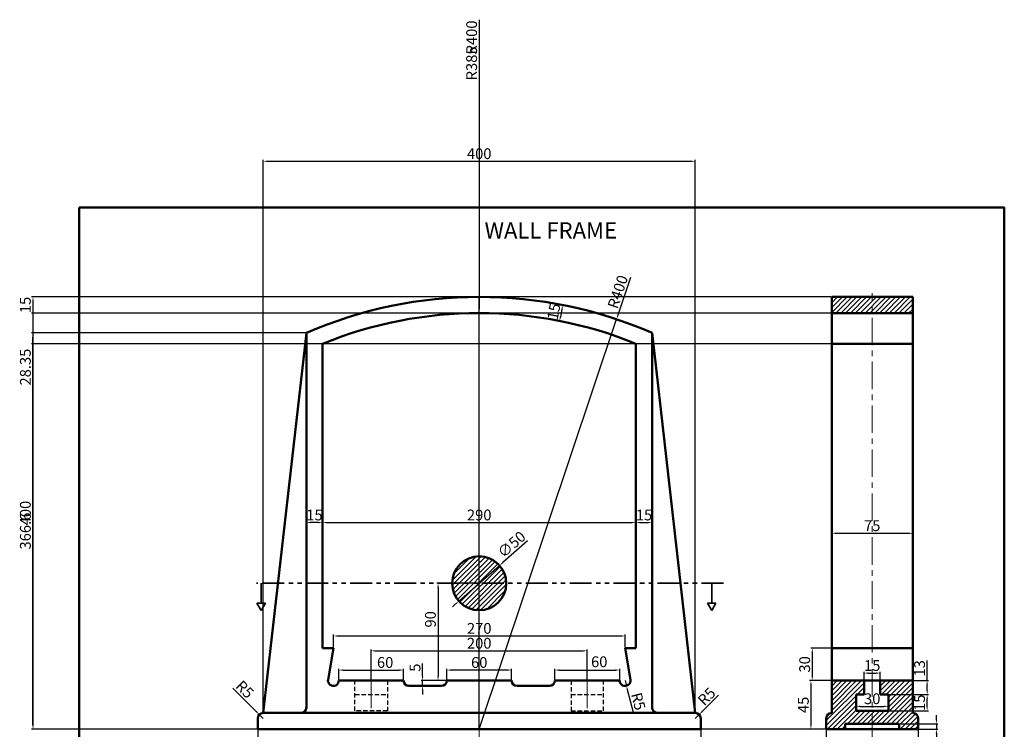
# Model space of a CAD drawing. Units: millimetres. Extents: x -150 to 761, y -175 to 827.
# Tile 2 of 2: x -150 to 761, y 171 to 827. Entities that reach past the tile are written whole.
import ezdxf

# ---------------------------------------------------------------- set-up
doc = ezdxf.new("R2010")
doc.units = ezdxf.units.MM
doc.header["$LTSCALE"] = 0.8
for name, pattern in [('CENTER', [50.8, 31.75, -6.35, 6.35, -6.35]), ('HIDDEN', [9.525, 6.35, -3.175]), ('PHANTOM', [63.5, 31.75, -6.35, 6.35, -6.35, 6.35, -6.35])]:
    doc.linetypes.add(name, pattern=pattern)
for name, color, linetype, lineweight in [('M-CNTR', 1, 'CENTER', 18), ('M-DIMS', 2, 'Continuous', 25), ('M-HATC', 8, 'Continuous', 18), ('M-HIDN', 4, 'HIDDEN', 25), ('M-OUTL', 7, 'Continuous', 50), ('M-SECT', 6, 'PHANTOM', 35), ('M-TEXT', 3, 'Continuous', 25), ('M-TTLB', 7, 'Continuous', 50)]:
    doc.layers.add(name, color=color, linetype=linetype, lineweight=lineweight)
doc.styles.get("Standard").update_dxf_attribs({"font": 'arial.ttf'})
doc.dimstyles.new('ISO-25', dxfattribs={"dimtxt": 10, "dimasz": 4, "dimexe": 1.25, "dimexo": 0.625, "dimtad": 1, "dimtxsty": 'Standard', "dimcen": 2.5, "dimadec": 0, "dimazin": 0, "dimtfac": 1, "dimtmove": 0, "dimatfit": 3, "dimfxl": 1, "dimarcsym": 0})

# ---------------------------------------------------------------- blocks, each defined once
blk = doc.blocks.new('*U1')
at = {"layer": 'M-CNTR', "color": 0, "transparency": 16777216}
blk.add_line((0, -217.92), (0, 196), dxfattribs=at)
blk = doc.blocks.new('*D2')
at = {"layer": 'Defpoints', "color": 0, "transparency": 16777216}
for p in [(646.18, 222.57), (631.18, 215.67), (646.18, 215.67)]:
    blk.add_point(p, dxfattribs=at)
at = {"layer": 'M-DIMS', "color": 0, "lineweight": -2, "transparency": 16777216}
for p, q in [((631.18, 216.29), (631.18, 223.82)), ((635.18, 222.57), (642.18, 222.57)), ((646.18, 216.29), (646.18, 223.82))]:
    blk.add_line(p, q, dxfattribs=at)
at = {"layer": 'M-DIMS', "color": 0, "transparency": 16777216}
for points in [[(635.18, 223.24), (635.18, 221.9), (631.18, 222.57)], [(642.18, 223.24), (642.18, 221.9), (646.18, 222.57)]]:
    blk.add_solid(points, dxfattribs=at)
at = {"layer": 'M-DIMS', "color": 0, "transparency": 16777216, "insert": (638.68, 228.3), "char_height": 10, "attachment_point": 5}
blk.add_mtext('15', dxfattribs=at)
blk = doc.blocks.new('*D3')
at = {"layer": 'Defpoints', "color": 0, "transparency": 16777216}
for p in [(623.68, 195.17), (653.68, 195.17), (653.68, 191.83)]:
    blk.add_point(p, dxfattribs=at)
at = {"layer": 'M-DIMS', "color": 0, "lineweight": -2, "transparency": 16777216}
for p, q in [((623.68, 194.54), (623.68, 190.58)), ((627.68, 191.83), (649.68, 191.83)), ((653.68, 194.54), (653.68, 190.58))]:
    blk.add_line(p, q, dxfattribs=at)
at = {"layer": 'M-DIMS', "color": 0, "transparency": 16777216}
for points in [[(627.68, 192.49), (627.68, 191.16), (623.68, 191.83)], [(649.68, 192.49), (649.68, 191.16), (653.68, 191.83)]]:
    blk.add_solid(points, dxfattribs=at)
at = {"layer": 'M-DIMS', "color": 0, "transparency": 16777216, "insert": (638.68, 197.56), "char_height": 10, "attachment_point": 5}
blk.add_mtext('30', dxfattribs=at)
blk = doc.blocks.new('*D4')
at = {"layer": 'Defpoints', "color": 0, "transparency": 16777216}
for p in [(601.18, 351.92), (676.18, 351.92), (676.18, 351.92)]:
    blk.add_point(p, dxfattribs=at)
at = {"layer": 'M-DIMS', "color": 0, "lineweight": -2, "transparency": 16777216}
for p, q in [((601.18, 352.54), (601.18, 353.17)), ((605.18, 351.92), (672.18, 351.92)), ((676.18, 352.54), (676.18, 353.17))]:
    blk.add_line(p, q, dxfattribs=at)
at = {"layer": 'M-DIMS', "color": 0, "transparency": 16777216}
for points in [[(605.18, 352.59), (605.18, 351.25), (601.18, 351.92)], [(672.18, 352.59), (672.18, 351.25), (676.18, 351.92)]]:
    blk.add_solid(points, dxfattribs=at)
at = {"layer": 'M-DIMS', "color": 0, "transparency": 16777216, "insert": (638.68, 357.63), "char_height": 10, "attachment_point": 5}
blk.add_mtext('75', dxfattribs=at)
blk = doc.blocks.new('*D5')
at = {"layer": 'Defpoints', "color": 0, "transparency": 16777216}
for p in [(601.18, 245.67), (583.18, 215.67), (601.18, 215.67)]:
    blk.add_point(p, dxfattribs=at)
at = {"layer": 'M-DIMS', "color": 0, "lineweight": -2, "transparency": 16777216}
for p, q in [((600.55, 245.67), (581.93, 245.67)), ((583.18, 241.67), (583.18, 219.67)), ((600.55, 215.67), (581.93, 215.67))]:
    blk.add_line(p, q, dxfattribs=at)
at = {"layer": 'M-DIMS', "color": 0, "transparency": 16777216}
for points in [[(582.52, 241.67), (583.85, 241.67), (583.18, 245.67)], [(582.52, 219.67), (583.85, 219.67), (583.18, 215.67)]]:
    blk.add_solid(points, dxfattribs=at)
at = {"layer": 'M-DIMS', "color": 0, "transparency": 16777216, "insert": (577.45, 230.67), "char_height": 10, "attachment_point": 5, "rotation": 90}
blk.add_mtext('30', dxfattribs=at)
blk = doc.blocks.new('*D6')
at = {"layer": 'Defpoints', "color": 0, "transparency": 16777216}
for p in [(591.24, 215.67), (581.93, 170.67), (596.18, 170.67)]:
    blk.add_point(p, dxfattribs=at)
at = {"layer": 'M-DIMS', "color": 0, "lineweight": -2, "transparency": 16777216}
for p, q in [((590.62, 215.67), (580.68, 215.67)), ((581.93, 211.67), (581.93, 174.67)), ((595.55, 170.67), (580.68, 170.67))]:
    blk.add_line(p, q, dxfattribs=at)
at = {"layer": 'M-DIMS', "color": 0, "transparency": 16777216}
for points in [[(581.27, 211.67), (582.6, 211.67), (581.93, 215.67)], [(581.27, 174.67), (582.6, 174.67), (581.93, 170.67)]]:
    blk.add_solid(points, dxfattribs=at)
at = {"layer": 'M-DIMS', "color": 0, "transparency": 16777216, "insert": (576.22, 193.17), "char_height": 10, "attachment_point": 5, "rotation": 90}
blk.add_mtext('45', dxfattribs=at)
blk = doc.blocks.new('*D7')
at = {"layer": 'Defpoints', "color": 0, "transparency": 16777216}
for p in [(653, 215.67), (653.68, 202.67), (689.52, 202.67)]:
    blk.add_point(p, dxfattribs=at)
at = {"layer": 'M-DIMS', "color": 0, "lineweight": -2, "transparency": 16777216}
for p, q in [((689.52, 215.67), (689.52, 234.3)), ((653.63, 215.67), (690.77, 215.67)), ((689.52, 206.67), (689.52, 211.67)), ((654.3, 202.67), (690.77, 202.67))]:
    blk.add_line(p, q, dxfattribs=at)
at = {"layer": 'M-DIMS', "color": 0, "transparency": 16777216}
for points in [[(688.86, 211.67), (690.19, 211.67), (689.52, 215.67)], [(688.86, 206.67), (690.19, 206.67), (689.52, 202.67)]]:
    blk.add_solid(points, dxfattribs=at)
at = {"layer": 'M-DIMS', "color": 0, "transparency": 16777216, "insert": (683.79, 226.99), "char_height": 10, "attachment_point": 5, "rotation": 90}
blk.add_mtext('13', dxfattribs=at)
blk = doc.blocks.new('*D8')
at = {"layer": 'Defpoints', "color": 0, "transparency": 16777216}
for p in [(653.68, 202.67), (689.52, 202.67), (653.68, 187.67)]:
    blk.add_point(p, dxfattribs=at)
at = {"layer": 'M-DIMS', "color": 0, "lineweight": -2, "transparency": 16777216}
for p, q in [((654.3, 202.67), (690.77, 202.67)), ((689.52, 191.67), (689.52, 198.67)), ((654.3, 187.67), (690.77, 187.67))]:
    blk.add_line(p, q, dxfattribs=at)
at = {"layer": 'M-DIMS', "color": 0, "transparency": 16777216}
for points in [[(688.86, 198.67), (690.19, 198.67), (689.52, 202.67)], [(688.86, 191.67), (690.19, 191.67), (689.52, 187.67)]]:
    blk.add_solid(points, dxfattribs=at)
at = {"layer": 'M-DIMS', "color": 0, "transparency": 16777216, "insert": (683.79, 195.17), "char_height": 10, "attachment_point": 5, "rotation": 90}
blk.add_mtext('15', dxfattribs=at)
blk = doc.blocks.new('*D9')
at = {"layer": 'Defpoints', "color": 0, "transparency": 16777216}
for p in [(663.68, 175.67), (663.68, 170.67), (698.09, 170.67)]:
    blk.add_point(p, dxfattribs=at)
at = {"layer": 'M-DIMS', "color": 0, "lineweight": -2, "transparency": 16777216}
for p, q in [((698.09, 179.67), (698.09, 183.67)), ((664.3, 175.67), (699.34, 175.67)), ((698.09, 175.67), (698.09, 170.67)), ((664.3, 170.67), (699.34, 170.67)), ((698.09, 166.67), (698.09, 154.79))]:
    blk.add_line(p, q, dxfattribs=at)
at = {"layer": 'M-DIMS', "color": 0, "transparency": 16777216}
for points in [[(697.42, 179.67), (698.75, 179.67), (698.09, 175.67)], [(697.42, 166.67), (698.75, 166.67), (698.09, 170.67)]]:
    blk.add_solid(points, dxfattribs=at)
at = {"layer": 'M-DIMS', "color": 0, "transparency": 16777216, "insert": (692.38, 158.73), "char_height": 10, "attachment_point": 5, "rotation": 90}
blk.add_mtext('5', dxfattribs=at)
blk = doc.blocks.new('*D11')
at = {"layer": 'Defpoints', "color": 0, "transparency": 16777216}
for p in [(596.18, 170.67), (681.18, 170.67), (596.18, 134.79)]:
    blk.add_point(p, dxfattribs=at)
at = {"layer": 'M-DIMS', "color": 0, "lineweight": -2, "transparency": 16777216}
for p, q in [((596.18, 170.04), (596.18, 133.54)), ((681.18, 170.04), (681.18, 133.54)), ((677.18, 134.79), (600.18, 134.79))]:
    blk.add_line(p, q, dxfattribs=at)
at = {"layer": 'M-DIMS', "color": 0, "transparency": 16777216}
for points in [[(600.18, 135.45), (600.18, 134.12), (596.18, 134.79)], [(677.18, 135.45), (677.18, 134.12), (681.18, 134.79)]]:
    blk.add_solid(points, dxfattribs=at)
at = {"layer": 'M-DIMS', "color": 0, "transparency": 16777216, "insert": (638.68, 140.52), "char_height": 10, "attachment_point": 5}
blk.add_mtext('85', dxfattribs=at)
blk = doc.blocks.new('*D12')
at = {"layer": 'Defpoints', "color": 0, "transparency": 16777216}
for p in [(419.95, 361.84), (129.95, 245.67), (419.95, 245.67)]:
    blk.add_point(p, dxfattribs=at)
at = {"layer": 'M-DIMS', "color": 0, "lineweight": -2, "transparency": 16777216}
for p, q in [((129.95, 246.29), (129.95, 363.09)), ((133.95, 361.84), (415.95, 361.84)), ((419.95, 246.29), (419.95, 363.09))]:
    blk.add_line(p, q, dxfattribs=at)
at = {"layer": 'M-DIMS', "color": 0, "transparency": 16777216}
for points in [[(133.95, 362.5), (133.95, 361.17), (129.95, 361.84)], [(415.95, 362.5), (415.95, 361.17), (419.95, 361.84)]]:
    blk.add_solid(points, dxfattribs=at)
at = {"layer": 'M-DIMS', "color": 0, "transparency": 16777216, "insert": (274.95, 367.57), "char_height": 10, "attachment_point": 5}
blk.add_mtext('290', dxfattribs=at)
blk = doc.blocks.new('*D13')
at = {"layer": 'Defpoints', "color": 0, "ltscale": 0.8, "transparency": 16777216}
for p in [(204.95, 225.38), (144.95, 215.67), (204.95, 215.67)]:
    blk.add_point(p, dxfattribs=at)
at = {"layer": 'M-DIMS', "color": 0, "lineweight": -2, "ltscale": 0.8, "transparency": 16777216}
for p, q in [((144.95, 216.29), (144.95, 226.63)), ((148.95, 225.38), (200.95, 225.38)), ((204.95, 216.29), (204.95, 226.63))]:
    blk.add_line(p, q, dxfattribs=at)
at = {"layer": 'M-DIMS', "color": 0, "ltscale": 0.8, "transparency": 16777216}
for points in [[(148.95, 226.05), (148.95, 224.71), (144.95, 225.38)], [(200.95, 226.05), (200.95, 224.71), (204.95, 225.38)]]:
    blk.add_solid(points, dxfattribs=at)
at = {"layer": 'M-DIMS', "color": 0, "ltscale": 0.8, "transparency": 16777216, "insert": (187.88, 231.11), "char_height": 10, "attachment_point": 5}
blk.add_mtext('60', dxfattribs=at)
blk = doc.blocks.new('*D14')
at = {"layer": 'Defpoints', "color": 0, "ltscale": 0.8, "transparency": 16777216}
for p in [(409.95, 256.93), (139.95, 245.67), (409.95, 245.67)]:
    blk.add_point(p, dxfattribs=at)
at = {"layer": 'M-DIMS', "color": 0, "lineweight": -2, "ltscale": 0.8, "transparency": 16777216}
for p, q in [((139.95, 246.29), (139.95, 258.18)), ((143.95, 256.93), (405.95, 256.93)), ((409.95, 246.29), (409.95, 258.18))]:
    blk.add_line(p, q, dxfattribs=at)
at = {"layer": 'M-DIMS', "color": 0, "ltscale": 0.8, "transparency": 16777216}
for points in [[(143.95, 257.6), (143.95, 256.27), (139.95, 256.93)], [(405.95, 257.6), (405.95, 256.27), (409.95, 256.93)]]:
    blk.add_solid(points, dxfattribs=at)
at = {"layer": 'M-DIMS', "color": 0, "ltscale": 0.8, "transparency": 16777216, "insert": (274.95, 262.66), "char_height": 10, "attachment_point": 5}
blk.add_mtext('270', dxfattribs=at)
blk = doc.blocks.new('*D15')
at = {"layer": 'Defpoints', "color": 0, "ltscale": 0.8, "transparency": 16777216}
for p in [(404.95, 225.38), (344.95, 215.67), (404.95, 215.67)]:
    blk.add_point(p, dxfattribs=at)
at = {"layer": 'M-DIMS', "color": 0, "lineweight": -2, "ltscale": 0.8, "transparency": 16777216}
for p, q in [((344.95, 216.29), (344.95, 226.63)), ((348.95, 225.38), (400.95, 225.38)), ((404.95, 216.29), (404.95, 226.63))]:
    blk.add_line(p, q, dxfattribs=at)
at = {"layer": 'M-DIMS', "color": 0, "ltscale": 0.8, "transparency": 16777216}
for points in [[(348.95, 226.05), (348.95, 224.71), (344.95, 225.38)], [(400.95, 226.05), (400.95, 224.71), (404.95, 225.38)]]:
    blk.add_solid(points, dxfattribs=at)
at = {"layer": 'M-DIMS', "color": 0, "ltscale": 0.8, "transparency": 16777216, "insert": (386.01, 231.76), "char_height": 10, "attachment_point": 5}
blk.add_mtext('60', dxfattribs=at)
blk = doc.blocks.new('*D16')
at = {"layer": 'Defpoints', "color": 0, "ltscale": 0.8, "transparency": 16777216}
for p in [(244.95, 225.38), (244.95, 215.67), (304.95, 215.67)]:
    blk.add_point(p, dxfattribs=at)
at = {"layer": 'M-DIMS', "color": 0, "lineweight": -2, "ltscale": 0.8, "transparency": 16777216}
for p, q in [((244.95, 216.29), (244.95, 226.63)), ((300.95, 225.38), (248.95, 225.38)), ((304.95, 216.29), (304.95, 226.63))]:
    blk.add_line(p, q, dxfattribs=at)
at = {"layer": 'M-DIMS', "color": 0, "ltscale": 0.8, "transparency": 16777216}
for points in [[(248.95, 226.05), (248.95, 224.71), (244.95, 225.38)], [(300.95, 226.05), (300.95, 224.71), (304.95, 225.38)]]:
    blk.add_solid(points, dxfattribs=at)
at = {"layer": 'M-DIMS', "color": 0, "ltscale": 0.8, "transparency": 16777216, "insert": (274.95, 231.11), "char_height": 10, "attachment_point": 5}
blk.add_mtext('60', dxfattribs=at)
blk = doc.blocks.new('*D17')
at = {"layer": 'Defpoints', "color": 0, "ltscale": 0.8, "transparency": 16777216}
for p in [(222.55, 215.67), (224.95, 210.67), (252.9, 215.67)]:
    blk.add_point(p, dxfattribs=at)
at = {"layer": 'M-DIMS', "color": 0, "lineweight": -2, "ltscale": 0.8, "transparency": 16777216}
for p, q in [((222.55, 219.67), (222.55, 231.55)), ((252.27, 215.67), (221.3, 215.67)), ((224.33, 210.67), (221.3, 210.67)), ((222.55, 210.67), (222.55, 215.67)), ((222.55, 206.67), (222.55, 202.67))]:
    blk.add_line(p, q, dxfattribs=at)
at = {"layer": 'M-DIMS', "color": 0, "ltscale": 0.8, "transparency": 16777216}
for points in [[(221.89, 219.67), (223.22, 219.67), (222.55, 215.67)], [(221.89, 206.67), (223.22, 206.67), (222.55, 210.67)]]:
    blk.add_solid(points, dxfattribs=at)
at = {"layer": 'M-DIMS', "color": 0, "ltscale": 0.8, "transparency": 16777216, "insert": (216.84, 227.61), "char_height": 10, "attachment_point": 5, "rotation": 90}
blk.add_mtext('5', dxfattribs=at)
blk = doc.blocks.new('*D18')
at = {"layer": 'Defpoints', "color": 0, "ltscale": 0.8, "transparency": 16777216}
for p in [(374.95, 243.16), (174.95, 215.67), (374.95, 215.67)]:
    blk.add_point(p, dxfattribs=at)
at = {"layer": 'M-DIMS', "color": 0, "lineweight": -2, "ltscale": 0.8, "transparency": 16777216}
for p, q in [((174.95, 216.29), (174.95, 244.41)), ((178.95, 243.16), (370.95, 243.16)), ((374.95, 216.29), (374.95, 244.41))]:
    blk.add_line(p, q, dxfattribs=at)
at = {"layer": 'M-DIMS', "color": 0, "ltscale": 0.8, "transparency": 16777216}
for points in [[(178.95, 243.83), (178.95, 242.5), (174.95, 243.16)], [(370.95, 243.83), (370.95, 242.5), (374.95, 243.16)]]:
    blk.add_solid(points, dxfattribs=at)
at = {"layer": 'M-DIMS', "color": 0, "ltscale": 0.8, "transparency": 16777216, "insert": (274.95, 248.9), "char_height": 10, "attachment_point": 5}
blk.add_mtext('200', dxfattribs=at)
blk = doc.blocks.new('*D19')
at = {"layer": 'Defpoints', "color": 0, "ltscale": 0.8, "transparency": 16777216}
for p in [(69.95, 170.67), (479.95, 170.67), (479.95, 149.01)]:
    blk.add_point(p, dxfattribs=at)
at = {"layer": 'M-DIMS', "color": 0, "lineweight": -2, "ltscale": 0.8, "transparency": 16777216}
for p, q in [((69.95, 170.04), (69.95, 147.76)), ((479.95, 170.04), (479.95, 147.76)), ((73.95, 149.01), (475.95, 149.01))]:
    blk.add_line(p, q, dxfattribs=at)
at = {"layer": 'M-DIMS', "color": 0, "ltscale": 0.8, "transparency": 16777216}
for points in [[(73.95, 149.68), (73.95, 148.35), (69.95, 149.01)], [(475.95, 149.68), (475.95, 148.35), (479.95, 149.01)]]:
    blk.add_solid(points, dxfattribs=at)
at = {"layer": 'M-DIMS', "color": 0, "ltscale": 0.8, "transparency": 16777216, "insert": (274.95, 154.74), "char_height": 10, "attachment_point": 5}
blk.add_mtext('410', dxfattribs=at)
blk = doc.blocks.new('*D20')
at = {"layer": 'Defpoints', "color": 0, "ltscale": 0.8, "transparency": 16777216}
for p in [(71.42, 184.21), (74.95, 180.67)]:
    blk.add_point(p, dxfattribs=at)
at = {"layer": 'M-DIMS', "color": 0, "lineweight": -2, "ltscale": 0.8, "transparency": 16777216}
for p, q in [((46.91, 208.75), (68.59, 187.04)), ((74.95, 180.67), (71.42, 184.21))]:
    blk.add_line(p, q, dxfattribs=at)
at = {"layer": 'M-DIMS', "color": 0, "ltscale": 0.8, "transparency": 16777216}
blk.add_solid([(69.06, 187.51), (68.12, 186.57), (71.42, 184.21)], dxfattribs=at)
at = {"layer": 'M-DIMS', "color": 0, "ltscale": 0.8, "transparency": 16777216, "insert": (57.11, 206.61), "char_height": 10, "attachment_point": 5, "rotation": 314.96518}
blk.add_mtext('R5', dxfattribs=at)
blk = doc.blocks.new('*D21')
at = {"layer": 'Defpoints', "color": 0, "ltscale": 0.8, "transparency": 16777216}
for p in [(409.95, 215.67), (411.22, 210.83)]:
    blk.add_point(p, dxfattribs=at)
at = {"layer": 'M-DIMS', "color": 0, "lineweight": -2, "ltscale": 0.8, "transparency": 16777216}
for p, q in [((409.95, 215.67), (411.22, 210.83)), ((417.69, 186.22), (412.24, 206.96))]:
    blk.add_line(p, q, dxfattribs=at)
at = {"layer": 'M-DIMS', "color": 0, "ltscale": 0.8, "transparency": 16777216}
blk.add_solid([(412.88, 207.13), (411.59, 206.8), (411.22, 210.83)], dxfattribs=at)
at = {"layer": 'M-DIMS', "color": 0, "ltscale": 0.8, "transparency": 16777216, "insert": (420.99, 196.11), "char_height": 10, "attachment_point": 5, "rotation": 284.72155}
blk.add_mtext('R5', dxfattribs=at)
blk = doc.blocks.new('*D22')
at = {"layer": 'Defpoints', "color": 0, "ltscale": 0.8, "transparency": 16777216}
for p in [(293.75, 322.15), (256.15, 289.19)]:
    blk.add_point(p, dxfattribs=at)
at = {"layer": 'M-DIMS', "color": 0, "lineweight": -2, "ltscale": 0.8, "transparency": 16777216}
for p, q in [((319.63, 344.84), (296.76, 324.79)), ((256.15, 289.19), (293.75, 322.15)), ((253.14, 286.55), (250.13, 283.92))]:
    blk.add_line(p, q, dxfattribs=at)
at = {"layer": 'M-DIMS', "color": 0, "ltscale": 0.8, "transparency": 16777216}
for points in [[(296.32, 325.29), (297.2, 324.28), (293.75, 322.15)], [(252.7, 287.05), (253.58, 286.05), (256.15, 289.19)]]:
    blk.add_solid(points, dxfattribs=at)
at = {"layer": 'M-DIMS', "color": 0, "ltscale": 0.8, "transparency": 16777216, "insert": (305.74, 340.65), "char_height": 10, "attachment_point": 5, "rotation": 41.23738}
blk.add_mtext('∅50', dxfattribs=at)
blk = doc.blocks.new('*D23')
at = {"layer": 'Defpoints', "color": 0, "ltscale": 0.8, "transparency": 16777216}
for p in [(274.95, 305.67), (236.84, 215.67), (274.95, 215.67)]:
    blk.add_point(p, dxfattribs=at)
at = {"layer": 'M-DIMS', "color": 0, "lineweight": -2, "ltscale": 0.8, "transparency": 16777216}
for p, q in [((274.33, 305.67), (235.59, 305.67)), ((236.84, 301.67), (236.84, 219.67)), ((274.33, 215.67), (235.59, 215.67))]:
    blk.add_line(p, q, dxfattribs=at)
at = {"layer": 'M-DIMS', "color": 0, "ltscale": 0.8, "transparency": 16777216}
for points in [[(236.17, 301.67), (237.5, 301.67), (236.84, 305.67)], [(236.17, 219.67), (237.5, 219.67), (236.84, 215.67)]]:
    blk.add_solid(points, dxfattribs=at)
at = {"layer": 'M-DIMS', "color": 0, "ltscale": 0.8, "transparency": 16777216, "insert": (231.1, 272.32), "char_height": 10, "attachment_point": 5, "rotation": 90}
blk.add_mtext('90', dxfattribs=at)
blk = doc.blocks.new('*D24')
at = {"layer": 'Defpoints', "color": 0, "ltscale": 0.8, "transparency": 16777216}
for p in [(114.95, 361.84), (114.95, 361.84), (129.95, 361.84)]:
    blk.add_point(p, dxfattribs=at)
at = {"layer": 'M-DIMS', "color": 0, "lineweight": -2, "ltscale": 0.8, "transparency": 16777216}
for p, q in [((114.95, 362.46), (114.95, 363.09)), ((125.95, 361.84), (118.95, 361.84)), ((129.95, 362.46), (129.95, 363.09))]:
    blk.add_line(p, q, dxfattribs=at)
at = {"layer": 'M-DIMS', "color": 0, "ltscale": 0.8, "transparency": 16777216}
for points in [[(118.95, 362.5), (118.95, 361.17), (114.95, 361.84)], [(125.95, 362.5), (125.95, 361.17), (129.95, 361.84)]]:
    blk.add_solid(points, dxfattribs=at)
at = {"layer": 'M-DIMS', "color": 0, "ltscale": 0.8, "transparency": 16777216, "insert": (122.45, 367.57), "char_height": 10, "attachment_point": 5}
blk.add_mtext('15', dxfattribs=at)
blk = doc.blocks.new('*D25')
at = {"layer": 'Defpoints', "color": 0, "ltscale": 0.8, "transparency": 16777216}
for p in [(419.95, 361.84), (434.95, 361.84), (434.95, 361.84)]:
    blk.add_point(p, dxfattribs=at)
at = {"layer": 'M-DIMS', "color": 0, "lineweight": -2, "ltscale": 0.8, "transparency": 16777216}
for p, q in [((419.95, 362.46), (419.95, 363.09)), ((423.95, 361.84), (430.95, 361.84)), ((434.95, 362.46), (434.95, 363.09))]:
    blk.add_line(p, q, dxfattribs=at)
at = {"layer": 'M-DIMS', "color": 0, "ltscale": 0.8, "transparency": 16777216}
for points in [[(423.95, 362.5), (423.95, 361.17), (419.95, 361.84)], [(430.95, 362.5), (430.95, 361.17), (434.95, 361.84)]]:
    blk.add_solid(points, dxfattribs=at)
at = {"layer": 'M-DIMS', "color": 0, "ltscale": 0.8, "transparency": 16777216, "insert": (427.45, 367.57), "char_height": 10, "attachment_point": 5}
blk.add_mtext('15', dxfattribs=at)
blk = doc.blocks.new('*D26')
at = {"layer": 'Defpoints', "color": 0, "ltscale": 0.8, "transparency": 16777216}
for p in [(402.06, 549.94), (274.95, 170.67)]:
    blk.add_point(p, dxfattribs=at)
at = {"layer": 'M-DIMS', "color": 0, "lineweight": -2, "ltscale": 0.8, "transparency": 16777216}
for p, q in [((415.05, 588.7), (403.33, 553.73)), ((274.95, 170.67), (402.06, 549.94))]:
    blk.add_line(p, q, dxfattribs=at)
at = {"layer": 'M-DIMS', "color": 0, "ltscale": 0.8, "transparency": 16777216}
blk.add_solid([(402.7, 553.94), (403.96, 553.52), (402.06, 549.94)], dxfattribs=at)
at = {"layer": 'M-DIMS', "color": 0, "ltscale": 0.8, "transparency": 16777216, "insert": (404.39, 574.93), "char_height": 10, "attachment_point": 5, "rotation": 71.47148}
blk.add_mtext('R400', dxfattribs=at)
blk = doc.blocks.new('*D27')
at = {"layer": 'Defpoints', "color": 0, "ltscale": 0.8, "transparency": 16777216}
for p in [(352.32, 563.12), (349.42, 548.4), (349.42, 548.4)]:
    blk.add_point(p, dxfattribs=at)
at = {"layer": 'M-DIMS', "color": 0, "lineweight": -2, "ltscale": 0.8, "transparency": 16777216}
for p, q in [((351.55, 559.19), (350.19, 552.32)), ((351.71, 563.24), (351.09, 563.36)), ((348.81, 548.52), (348.19, 548.64))]:
    blk.add_line(p, q, dxfattribs=at)
at = {"layer": 'M-DIMS', "color": 0, "ltscale": 0.8, "transparency": 16777216}
for points in [[(350.89, 559.32), (352.2, 559.06), (352.32, 563.12)], [(349.54, 552.45), (350.85, 552.19), (349.42, 548.4)]]:
    blk.add_solid(points, dxfattribs=at)
at = {"layer": 'M-DIMS', "color": 0, "ltscale": 0.8, "transparency": 16777216, "insert": (345.25, 556.87), "char_height": 10, "attachment_point": 5, "rotation": 78.84725}
blk.add_mtext('15', dxfattribs=at)
blk = doc.blocks.new('*D47')
at = {"layer": 'Defpoints', "color": 0, "ltscale": 0.8, "transparency": 16777216}
for p in [(-138.06, 537.28), (114.95, 537.28), (69.95, 170.67)]:
    blk.add_point(p, dxfattribs=at)
at = {"layer": 'M-DIMS', "color": 0, "lineweight": -2, "ltscale": 0.8, "transparency": 16777216}
for p, q in [((114.33, 537.28), (-139.31, 537.28)), ((-138.06, 174.67), (-138.06, 533.28)), ((69.33, 170.67), (-139.31, 170.67))]:
    blk.add_line(p, q, dxfattribs=at)
at = {"layer": 'M-DIMS', "color": 0, "ltscale": 0.8, "transparency": 16777216}
for points in [[(-138.72, 533.28), (-137.39, 533.28), (-138.06, 537.28)], [(-138.72, 174.67), (-137.39, 174.67), (-138.06, 170.67)]]:
    blk.add_solid(points, dxfattribs=at)
at = {"layer": 'M-DIMS', "color": 0, "ltscale": 0.8, "transparency": 16777216, "insert": (-143.79, 353.97), "char_height": 10, "attachment_point": 5, "rotation": 90}
blk.add_mtext('366.6', dxfattribs=at)
blk = doc.blocks.new('*D48')
at = {"layer": 'Defpoints', "color": 0, "ltscale": 0.8, "transparency": 16777216}
for p in [(474.95, 696.11), (74.95, 185.67), (474.95, 185.67)]:
    blk.add_point(p, dxfattribs=at)
at = {"layer": 'M-DIMS', "color": 0, "lineweight": -2, "ltscale": 0.8, "transparency": 16777216}
for p, q in [((74.95, 186.29), (74.95, 697.36)), ((78.95, 696.11), (470.95, 696.11)), ((474.95, 186.29), (474.95, 697.36))]:
    blk.add_line(p, q, dxfattribs=at)
at = {"layer": 'M-DIMS', "color": 0, "ltscale": 0.8, "transparency": 16777216}
for points in [[(78.95, 696.77), (78.95, 695.44), (74.95, 696.11)], [(470.95, 696.77), (470.95, 695.44), (474.95, 696.11)]]:
    blk.add_solid(points, dxfattribs=at)
at = {"layer": 'M-DIMS', "color": 0, "ltscale": 0.8, "transparency": 16777216, "insert": (274.95, 701.84), "char_height": 10, "attachment_point": 5}
blk.add_mtext('400', dxfattribs=at)
blk = doc.blocks.new('*D49')
at = {"layer": 'Defpoints', "color": 0, "ltscale": 0.8, "transparency": 16777216}
for p in [(601.18, 570.67), (-138.06, 555.67), (601.18, 555.67)]:
    blk.add_point(p, dxfattribs=at)
at = {"layer": 'M-DIMS', "color": 0, "lineweight": -2, "ltscale": 0.8, "transparency": 16777216}
for p, q in [((600.55, 570.67), (-139.31, 570.67)), ((-138.06, 566.67), (-138.06, 559.67)), ((600.55, 555.67), (-139.31, 555.67))]:
    blk.add_line(p, q, dxfattribs=at)
at = {"layer": 'M-DIMS', "color": 0, "ltscale": 0.8, "transparency": 16777216}
for points in [[(-138.72, 566.67), (-137.39, 566.67), (-138.06, 570.67)], [(-138.72, 559.67), (-137.39, 559.67), (-138.06, 555.67)]]:
    blk.add_solid(points, dxfattribs=at)
at = {"layer": 'M-DIMS', "color": 0, "ltscale": 0.8, "transparency": 16777216, "insert": (-143.79, 563.17), "char_height": 10, "attachment_point": 5, "rotation": 90}
blk.add_mtext('15', dxfattribs=at)
blk = doc.blocks.new('*D50')
at = {"layer": 'Defpoints', "color": 0, "ltscale": 0.8, "transparency": 16777216}
for p in [(601.18, 555.67), (-138.06, 527.32), (601.18, 527.32)]:
    blk.add_point(p, dxfattribs=at)
at = {"layer": 'M-DIMS', "color": 0, "lineweight": -2, "ltscale": 0.8, "transparency": 16777216}
for p, q in [((600.55, 555.67), (-139.31, 555.67)), ((-138.06, 551.67), (-138.06, 531.32)), ((600.55, 527.32), (-139.31, 527.32)), ((-138.06, 527.32), (-138.06, 488.08))]:
    blk.add_line(p, q, dxfattribs=at)
at = {"layer": 'M-DIMS', "color": 0, "ltscale": 0.8, "transparency": 16777216}
for points in [[(-138.72, 551.67), (-137.39, 551.67), (-138.06, 555.67)], [(-138.72, 531.32), (-137.39, 531.32), (-138.06, 527.32)]]:
    blk.add_solid(points, dxfattribs=at)
at = {"layer": 'M-DIMS', "color": 0, "ltscale": 0.8, "transparency": 16777216, "insert": (-143.79, 505.7), "char_height": 10, "attachment_point": 5, "rotation": 90}
blk.add_mtext('28.35', dxfattribs=at)
blk = doc.blocks.new('*D51')
at = {"layer": 'Defpoints', "color": 0, "ltscale": 0.8, "transparency": 16777216}
for p in [(601.18, 570.67), (-138.06, 170.67), (596.18, 170.67)]:
    blk.add_point(p, dxfattribs=at)
at = {"layer": 'M-DIMS', "color": 0, "lineweight": -2, "ltscale": 0.8, "transparency": 16777216}
for p, q in [((600.55, 570.67), (-139.31, 570.67)), ((-138.06, 566.67), (-138.06, 174.67)), ((595.55, 170.67), (-139.31, 170.67))]:
    blk.add_line(p, q, dxfattribs=at)
at = {"layer": 'M-DIMS', "color": 0, "ltscale": 0.8, "transparency": 16777216}
for points in [[(-138.72, 566.67), (-137.39, 566.67), (-138.06, 570.67)], [(-138.72, 174.67), (-137.39, 174.67), (-138.06, 170.67)]]:
    blk.add_solid(points, dxfattribs=at)
at = {"layer": 'M-DIMS', "color": 0, "ltscale": 0.8, "transparency": 16777216, "insert": (-143.79, 370.67), "char_height": 10, "attachment_point": 5, "rotation": 90}
blk.add_mtext('400', dxfattribs=at)
blk = doc.blocks.new('*D52')
at = {"layer": 'Defpoints', "color": 0, "ltscale": 0.8, "transparency": 16777216}
for p in [(274.95, 570.67), (274.95, 170.67)]:
    blk.add_point(p, dxfattribs=at)
at = {"layer": 'M-DIMS', "color": 0, "lineweight": -2, "ltscale": 0.8, "transparency": 16777216}
for p, q in [((274.95, 827.11), (274.95, 574.67)), ((274.95, 170.67), (274.95, 570.67))]:
    blk.add_line(p, q, dxfattribs=at)
at = {"layer": 'M-DIMS', "color": 0, "ltscale": 0.8, "transparency": 16777216}
blk.add_solid([(274.28, 574.67), (275.62, 574.67), (274.95, 570.67)], dxfattribs=at)
at = {"layer": 'M-DIMS', "color": 0, "ltscale": 0.8, "transparency": 16777216, "insert": (269.22, 810.67), "char_height": 10, "attachment_point": 5, "rotation": 90}
blk.add_mtext('R400', dxfattribs=at)
blk = doc.blocks.new('*D53')
at = {"layer": 'Defpoints', "color": 0, "ltscale": 0.8, "transparency": 16777216}
for p in [(274.95, 555.67), (274.95, 170.67)]:
    blk.add_point(p, dxfattribs=at)
at = {"layer": 'M-DIMS', "color": 0, "lineweight": -2, "ltscale": 0.8, "transparency": 16777216}
for p, q in [((274.95, 803.16), (274.95, 559.67)), ((274.95, 170.67), (274.95, 555.67))]:
    blk.add_line(p, q, dxfattribs=at)
at = {"layer": 'M-DIMS', "color": 0, "ltscale": 0.8, "transparency": 16777216}
blk.add_solid([(274.28, 559.67), (275.62, 559.67), (274.95, 555.67)], dxfattribs=at)
at = {"layer": 'M-DIMS', "color": 0, "ltscale": 0.8, "transparency": 16777216, "insert": (269.22, 786.67), "char_height": 10, "attachment_point": 5, "rotation": 90}
blk.add_mtext('R385', dxfattribs=at)
blk = doc.blocks.new('*D56')
at = {"layer": 'Defpoints', "color": 0, "ltscale": 0.8, "transparency": 16777216}
for p in [(478.5, 184.2), (474.95, 180.67)]:
    blk.add_point(p, dxfattribs=at)
at = {"layer": 'M-DIMS', "color": 0, "lineweight": -2, "ltscale": 0.8, "transparency": 16777216}
for p, q in [((496.54, 202.14), (481.33, 187.02)), ((474.95, 180.67), (478.5, 184.2))]:
    blk.add_line(p, q, dxfattribs=at)
at = {"layer": 'M-DIMS', "color": 0, "ltscale": 0.8, "transparency": 16777216}
blk.add_solid([(480.86, 187.49), (481.8, 186.54), (478.5, 184.2)], dxfattribs=at)
at = {"layer": 'M-DIMS', "color": 0, "ltscale": 0.8, "transparency": 16777216, "insert": (486.33, 200.04), "char_height": 10, "attachment_point": 5, "rotation": 44.8446}
blk.add_mtext('R5', dxfattribs=at)

msp = doc.modelspace()

# ---------------------------------------------------------------- hatches: boundary and pattern name
at = {"layer": 'M-HATC'}
h = msp.add_hatch(dxfattribs=at)
h.set_pattern_fill('ANSI31', color=256)
h.paths.add_polyline_path([(676.178, 570.67), (638.678, 570.67), (638.678, 555.67), (676.178, 555.67)])
h.paths.add_polyline_path([(638.678, 570.67), (601.178, 570.67), (601.178, 555.67), (638.678, 555.67)])
at = {"layer": 'M-HATC', "ltscale": 0.8}
h = msp.add_hatch(dxfattribs=at)
h.set_pattern_fill('ANSI31', color=256)
h.paths.add_polyline_path([(274.95, 330.67), (274.95, 280.67, 0.4142136), (299.95, 305.67, 0.4142136)])
h.paths.add_polyline_path([(274.95, 330.67, 0.4142136), (249.95, 305.67, 0.4142136), (274.95, 280.67)])
at = {"layer": 'M-HATC'}
h = msp.add_hatch(dxfattribs=at)
h.set_pattern_fill('ANSI31', color=256)
h.paths.add_polyline_path([(623.678, 202.67), (631.178, 202.67), (631.178, 215.67), (601.178, 215.67), (601.178, 185.67, 0.4142136), (596.178, 180.67), (596.178, 170.67), (613.678, 170.67), (613.678, 175.67), (638.678, 175.67), (638.678, 187.67), (623.678, 187.67)])
h.paths.add_polyline_path([(653.678, 187.67), (638.678, 187.67), (638.678, 175.67), (663.678, 175.67), (663.678, 170.67), (681.178, 170.67), (681.178, 180.67, 0.4142136), (676.178, 185.67), (676.178, 215.67), (646.178, 215.67), (646.178, 202.67), (653.678, 202.67)])

# ---------------------------------------------------------------- linework, layer by layer
at = {"layer": 'M-CNTR'}
for p, q in [((274.95, -122.062), (274.95, 589.539)), ((174.95, 215.67), (174.95, 185.67)), ((204.95, 215.67), (204.95, 215.67)), ((344.95, 215.67), (344.95, 215.67)), ((374.95, 215.67), (374.95, 185.67))]:
    msp.add_line(p, q, dxfattribs=at)
at = {"layer": 'M-HIDN', "ltscale": 0.8}
for p, q in [((159.95, 187.67), (159.95, 215.67)), ((159.95, 215.67), (189.95, 215.67)), ((189.95, 215.67), (189.95, 187.67)), ((359.95, 215.67), (359.95, 187.67)), ((389.95, 215.67), (359.95, 215.67)), ((389.95, 187.67), (389.95, 215.67)), ((159.95, 202.67), (189.95, 202.67)), ((359.95, 202.67), (389.95, 202.67)), ((189.95, 187.67), (159.95, 187.67)), ((359.95, 187.67), (389.95, 187.67))]:
    msp.add_line(p, q, dxfattribs=at)
at = {"layer": 'M-OUTL'}
for p, q in [((601.178, 570.67), (676.178, 570.67)), ((601.178, 185.67), (601.178, 570.67)), ((676.178, 185.67), (676.178, 570.67)), ((601.178, 555.67), (676.178, 555.67)), ((114.95, 537.276), (74.95, 185.67)), ((114.95, 190.67), (114.95, 537.276)), ((434.95, 190.67), (434.95, 537.276)), ((434.95, 537.276), (474.95, 185.67)), ((129.95, 245.67), (129.95, 527.321)), ((419.95, 245.67), (419.95, 527.321)), ((601.178, 527.321), (676.178, 527.321)), ((129.95, 245.67), (139.95, 245.67)), ((409.95, 245.67), (419.95, 245.67)), ((601.178, 245.67), (676.178, 245.67)), ((244.95, 215.67), (244.95, 215.67)), ((244.95, 215.67), (304.95, 215.67)), ((304.95, 215.67), (304.95, 215.67)), ((601.178, 215.67), (676.178, 215.67)), ((631.178, 215.67), (631.178, 202.67)), ((646.178, 215.67), (631.178, 215.67)), ((646.178, 202.67), (646.178, 215.67)), ((631.178, 202.67), (623.678, 202.67)), ((623.678, 202.67), (623.678, 187.67)), ((653.678, 202.67), (646.178, 202.67)), ((653.678, 187.67), (653.678, 202.67)), ((474.95, 185.67), (74.95, 185.67)), ((601.178, 185.67), (601.178, 185.67)), ((623.678, 187.67), (653.678, 187.67)), ((676.178, 185.67), (676.178, 185.67)), ((69.95, 180.67), (69.95, 170.67)), ((479.95, 170.67), (479.95, 180.67)), ((596.178, 170.67), (596.178, 180.67)), ((613.678, 175.67), (613.678, 170.67)), ((663.678, 175.67), (613.678, 175.67)), ((663.678, 170.67), (663.678, 175.67)), ((681.178, 170.67), (681.178, 180.67)), ((69.95, 170.67), (479.95, 170.67)), ((596.178, 170.67), (681.178, 170.67)), ((613.678, 170.67), (663.678, 170.67))]:
    msp.add_line(p, q, dxfattribs=at)
at = {"layer": 'M-OUTL', "ltscale": 0.8}
for p, q in [((135.02, 216.503), (139.95, 245.67)), ((414.88, 216.503), (409.95, 245.67)), ((204.95, 215.67), (144.95, 215.67)), ((239.95, 210.67), (209.95, 210.67)), ((309.95, 210.67), (339.95, 210.67)), ((344.95, 215.67), (404.95, 215.67))]:
    msp.add_line(p, q, dxfattribs=at)
msp.add_circle((274.95, 305.67), 25, dxfattribs=at)
at = {"layer": 'M-OUTL'}
for centre, radius, start, end in [((274.95, 170.67), 400, 66.421822, 113.578178), ((274.95, 170.67), 385, 67.875317, 112.124683), ((239.95, 215.67), 5, 270, 0), ((74.95, 180.67), 5, 90, 180), ((474.95, 180.67), 5, 0, 90), ((601.178, 180.67), 5, 90, 180), ((676.178, 180.67), 5, 360, 90)]:
    msp.add_arc(centre, radius, start, end, dxfattribs=at)
at = {"layer": 'M-OUTL', "ltscale": 0.8}
for centre, start, end in [((139.95, 215.67), 170.405932, 0), ((209.95, 215.67), 180, 270), ((309.95, 215.67), 180, 270), ((339.95, 215.67), 270, 360), ((409.95, 215.67), 180, 9.594068), ((109.95, 190.67), 270, 0), ((439.95, 190.67), 180, 270)]:
    msp.add_arc(centre, 5, start, end, dxfattribs=at)
at = {"layer": 'M-SECT', "ltscale": 0.8}
for p, q in [((500.933, 305.67), (68.799, 305.67)), ((73.164, 305.67), (73.164, 287.389)), ((490.1, 305.67), (490.1, 287.389)), ((73.164, 280.632), (69.263, 287.389)), ((69.263, 287.389), (77.065, 287.389)), ((73.164, 280.632), (77.065, 287.389)), ((490.1, 280.632), (486.199, 287.389)), ((486.199, 287.389), (494.001, 287.389)), ((490.1, 280.632), (494.001, 287.389))]:
    msp.add_line(p, q, dxfattribs=at)
at = {"layer": 'M-TTLB', "ltscale": 0.8}
msp.add_lwpolyline([(-95.156, 653.208), (760.935, 653.208), (760.935, -175.003), (-95.156, -175.003)], close=True, dxfattribs=at)

# ---------------------------------------------------------------- block references
at = {"layer": 'M-CNTR'}
msp.add_blockref('*U1', (638.678, 378.17), dxfattribs=at)

# ---------------------------------------------------------------- texts
at = {"layer": 'M-TEXT', "ltscale": 0.8, "insert": (279.902, 639.67), "char_height": 15, "attachment_point": 1}
msp.add_mtext_dynamic_manual_height_columns('WALL FRAME', width=134.05729, gutter_width=12.5, heights=[12.09], dxfattribs=at)

# ---------------------------------------------------------------- dimensions: what is measured, and where the dimension line sits
at = {"layer": 'M-DIMS', "ltscale": 0.8}
for center, mpoint, override, picture, middle in [((274.95, 170.67), (274.95, 570.67), {"dimdec": 0, "dimlfac": 1, "dimrnd": 0, "dimzin": 0, "dimdsep": 46, "dimlunit": 2}, '*D52', (274.95, 810.67)), ((274.95, 170.67), (274.95, 555.67), {"dimdec": 0, "dimlfac": 1, "dimrnd": 0, "dimzin": 0, "dimdsep": 46, "dimlunit": 2}, '*D53', (274.95, 786.67)), ((74.95, 180.67), (71.417, 184.207), {"dimclrd": 0, "dimclre": 0, "dimclrt": 0}, '*D20', (53.075, 202.572))]:
    dim = msp.add_radius_dim(center=center, mpoint=mpoint, dimstyle='ISO-25', override=override, dxfattribs=at)
    dim.commit()
    dim.dimension.update_dxf_attribs({"geometry": picture, "text_midpoint": middle, "dimtype": 164})
for base, p1, p2, override, picture, middle in [((474.95, 696.108), (74.95, 185.67), (474.95, 185.67), {"dimdec": 0, "dimlfac": 1, "dimrnd": 0, "dimzin": 0, "dimdsep": 46, "dimlunit": 2}, '*D48', (274.95, 701.839)), ((114.95, 361.837), (129.95, 361.837), (114.95, 361.837), {"dimclrd": 0, "dimclre": 0, "dimclrt": 0}, '*D24', (122.45, 367.568)), ((434.95, 361.837), (419.95, 361.837), (434.95, 361.837), {"dimclrd": 0, "dimclre": 0, "dimclrt": 0}, '*D25', (427.45, 367.568)), ((409.95, 256.934), (139.95, 245.67), (409.95, 245.67), {"dimclrd": 0, "dimclre": 0, "dimclrt": 0}, '*D14', (274.95, 262.665)), ((374.95, 243.165), (174.95, 215.67), (374.95, 215.67), {"dimclrd": 0, "dimclre": 0, "dimclrt": 0}, '*D18', (274.95, 248.896)), ((479.95, 149.013), (69.95, 170.67), (479.95, 170.67), {"dimclrd": 0, "dimclre": 0, "dimclrt": 0}, '*D19', (274.95, 154.744))]:
    dim = msp.add_linear_dim(base=base, p1=p1, p2=p2, dimstyle='ISO-25', override=override, dxfattribs=at)
    dim.commit()
    dim.dimension.update_dxf_attribs({"geometry": picture, "text_midpoint": middle})
for center, mpoint, override, picture, middle in [((274.95, 170.67), (402.061, 549.936), {"dimclrd": 0, "dimclre": 0, "dimclrt": 0}, '*D26', (404.394, 574.93)), ((409.95, 215.67), (411.221, 210.834), {"dimclrd": 0, "dimclre": 0, "dimclrt": 0}, '*D21', (420.994, 196.109)), ((474.95, 180.67), (478.495, 184.195), {"dimdec": 0, "dimlfac": 1, "dimrnd": 0, "dimzin": 0, "dimdsep": 46, "dimlunit": 2}, '*D56', (486.327, 200.039))]:
    dim = msp.add_radius_dim(center=center, mpoint=mpoint, dimstyle='ISO-25', override=override, dxfattribs=at)
    dim.commit()
    dim.dimension.update_dxf_attribs({"geometry": picture, "text_midpoint": middle})
for base, p1, p2, override, picture, middle in [((-138.056, 555.67), (601.178, 570.67), (601.178, 555.67), {"dimdec": 0, "dimlfac": 1, "dimrnd": 0, "dimzin": 0, "dimdsep": 46, "dimlunit": 2}, '*D49', (-143.786, 563.17)), ((-138.056, 170.67), (601.178, 570.67), (596.178, 170.67), {"dimdec": 0, "dimlfac": 1, "dimrnd": 0, "dimzin": 0, "dimdsep": 46, "dimlunit": 2}, '*D51', (-143.786, 370.67)), ((-138.056, 527.321), (601.178, 555.67), (601.178, 527.321), {"dimdec": 2, "dimlfac": 1, "dimrnd": 0, "dimzin": 0, "dimdsep": 46, "dimlunit": 2}, '*D50', (-143.79, 505.7)), ((-138.056, 537.276), (69.95, 170.67), (114.95, 537.276), {"dimdec": 1, "dimlfac": 1, "dimrnd": 0, "dimzin": 0, "dimdsep": 46, "dimlunit": 2}, '*D47', (-143.79, 353.973)), ((222.552, 215.67), (224.95, 210.67), (252.9, 215.67), {"dimclrd": 0, "dimclre": 0, "dimclrt": 0}, '*D17', (216.842, 227.61))]:
    dim = msp.add_linear_dim(base=base, p1=p1, p2=p2, angle=90, dimstyle='ISO-25', override=override, dxfattribs=at)
    dim.commit()
    dim.dimension.update_dxf_attribs({"geometry": picture, "text_midpoint": middle})
dim = msp.add_aligned_dim(p1=(352.32, 563.116), p2=(349.419, 548.399), distance=0, dimstyle='ISO-25', override={"dimclrd": 0, "dimclre": 0, "dimclrt": 0}, dxfattribs=at)
dim.commit()
dim.dimension.update_dxf_attribs({"geometry": '*D27', "text_midpoint": (345.247, 556.866)})
at = {"layer": 'M-DIMS'}
dim = msp.add_linear_dim(base=(419.95, 361.837), p1=(129.95, 245.67), p2=(419.95, 245.67), dimstyle='ISO-25', override={"dimclrd": 0, "dimclre": 0, "dimclrt": 0}, dxfattribs=at)
dim.commit()
dim.dimension.update_dxf_attribs({"geometry": '*D12', "text_midpoint": (274.95, 361.837), "dimtype": 160})
for base, p1, p2, picture, middle in [((676.178, 351.919), (601.178, 351.919), (676.178, 351.919), '*D4', (638.678, 357.629)), ((646.178, 222.568), (631.178, 215.67), (646.178, 215.67), '*D2', (638.678, 228.299)), ((653.678, 191.825), (623.678, 195.17), (653.678, 195.17), '*D3', (638.678, 197.559)), ((596.178, 134.787), (681.178, 170.67), (596.178, 170.67), '*D11', (638.678, 140.518))]:
    dim = msp.add_linear_dim(base=base, p1=p1, p2=p2, dimstyle='ISO-25', override={"dimclrd": 0, "dimclre": 0, "dimclrt": 0}, dxfattribs=at)
    dim.commit()
    dim.dimension.update_dxf_attribs({"geometry": picture, "text_midpoint": middle})
at = {"layer": 'M-DIMS', "ltscale": 0.8}
dim = msp.add_diameter_dim_2p(p1=(256.151, 289.19), p2=(293.75, 322.149), dimstyle='ISO-25', override={"dimclrd": 0, "dimclre": 0, "dimclrt": 0}, dxfattribs=at)
dim.commit()
dim.dimension.update_dxf_attribs({"geometry": '*D22', "text_midpoint": (305.738, 340.65)})
dim = msp.add_linear_dim(base=(236.835, 215.67), p1=(274.95, 305.67), p2=(274.95, 215.67), angle=90, dimstyle='ISO-25', override={"dimclrd": 0, "dimclre": 0, "dimclrt": 0, "dimtmove": 2}, dxfattribs=at)
dim.commit()
dim.dimension.update_dxf_attribs({"geometry": '*D23', "text_midpoint": (231.105, 272.32), "dimtype": 160})
for base, p1, p2, override, picture, middle in [((204.95, 225.382), (144.95, 215.67), (204.95, 215.67), {"dimclrd": 0, "dimclre": 0, "dimclrt": 0, "dimtmove": 2}, '*D13', (187.881, 231.112)), ((244.95, 225.382), (304.95, 215.67), (244.95, 215.67), {"dimclrd": 0, "dimclre": 0, "dimclrt": 0, "dimtmove": 0}, '*D16', (274.95, 225.382)), ((404.95, 225.382), (344.95, 215.67), (404.95, 215.67), {"dimclrd": 0, "dimclre": 0, "dimclrt": 0, "dimtmove": 2}, '*D15', (386.006, 231.765))]:
    dim = msp.add_linear_dim(base=base, p1=p1, p2=p2, dimstyle='ISO-25', override=override, dxfattribs=at)
    dim.commit()
    dim.dimension.update_dxf_attribs({"geometry": picture, "text_midpoint": middle, "dimtype": 160})
at = {"layer": 'M-DIMS'}
for base, p1, p2, picture, middle in [((583.185, 215.67), (601.178, 245.67), (601.178, 215.67), '*D5', (577.451, 230.67)), ((581.935, 170.67), (591.244, 215.67), (596.178, 170.67), '*D6', (576.224, 193.17)), ((689.522, 202.67), (653.678, 187.67), (653.678, 202.67), '*D8', (683.791, 195.17)), ((698.087, 170.67), (663.678, 175.67), (663.678, 170.67), '*D9', (692.377, 158.729))]:
    dim = msp.add_linear_dim(base=base, p1=p1, p2=p2, angle=90, dimstyle='ISO-25', override={"dimclrd": 0, "dimclre": 0, "dimclrt": 0}, dxfattribs=at)
    dim.commit()
    dim.dimension.update_dxf_attribs({"geometry": picture, "text_midpoint": middle})
dim = msp.add_linear_dim(base=(689.522, 202.67), p1=(653.001, 215.67), p2=(653.678, 202.67), angle=90, dimstyle='ISO-25', override={"dimclrd": 0, "dimclre": 0, "dimclrt": 0}, dxfattribs=at)
dim.commit()
dim.dimension.update_dxf_attribs({"geometry": '*D7', "text_midpoint": (689.522, 226.986), "dimtype": 160})

doc.saveas('drawing.dxf')
